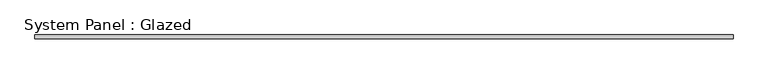
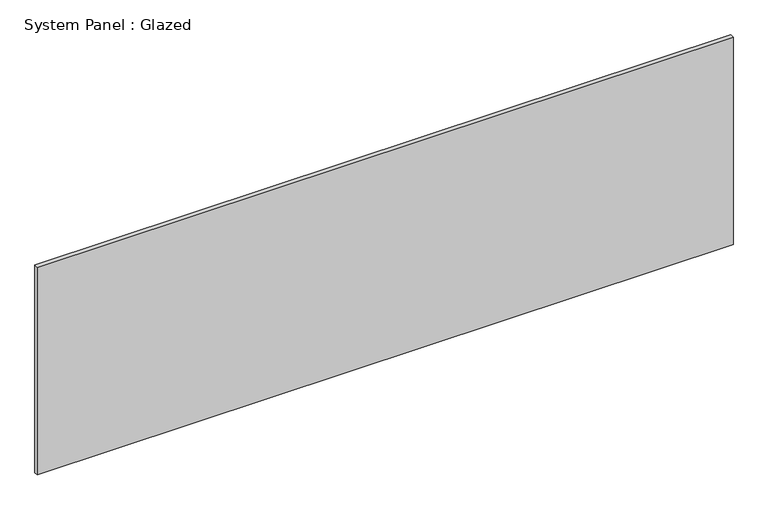
"""IFC4 building model written with IfcOpenShell, lengths in millimetres: plate geometry, System Panel : Glazed."""

from ifc_helpers import new_model, si_unit, origin, origin_with_axes, place, context, project, spatial, polyline, outline, extrude, source, transform, mapped, element, save


def system_panel_glazed_066de0f8(model_context):
    return source(origin(), model_context, "Body", "SweptSolid", [
        extrude(outline(polyline([(2315.343154, 19.05), (-2315.343154, 19.05), (-2315.343154, 44.45), (2315.343154, 44.45), (2315.343154, 19.05)])), origin_with_axes(), (0.0, 0.0, 1.0), 1460.5),
    ])


if __name__ == "__main__":
    model = new_model("IFC4")
    model_context = context("Model", 3, world=origin())
    ifc_project = project(units=[si_unit("LENGTHUNIT", "METRE", prefix="MILLI")], contexts=[model_context])
    site = spatial("IfcSite", under=ifc_project)
    building = spatial("IfcBuilding", under=site)
    placement = place(None, origin())
    system_panel_glazed_shape = system_panel_glazed_066de0f8(model_context)
    element("IfcPlate", 1, ObjectType="System Panel : Glazed", at=placement, inside=building, context=model_context, shape_type="MappedRepresentation", body=[
        mapped(system_panel_glazed_shape, transform((0.0, 0.0, 0.0), x_axis=(1.0, 0.0, 0.0), y_axis=(0.0, 1.0, 0.0), z_axis=(0.0, 0.0, 1.0))),
    ])
    save(model, "model.ifc")

# Revit data of these elements
# Type "System Panel : Glazed"
#   Construction Type Id = "GSP4R"
#   Analytic Construction = "1/8 in Pilkington single glazing"
#   Visual Light Transmittance = 0.9
#   Solar Heat Gain Coefficient = 0.86
#   Heat Transfer Coefficient (U) = 1.18115 BTU/(h·ft²·°F)
# Element 1 (IfcPlate, "System Panel : Glazed")
#   Materials on its faces: "Glass"
# Materials
#   "Glass": class "Glass", colour RGB 0 128 192, transparency 0.75, Description = "Soda Lime Glass", Cost = 0
